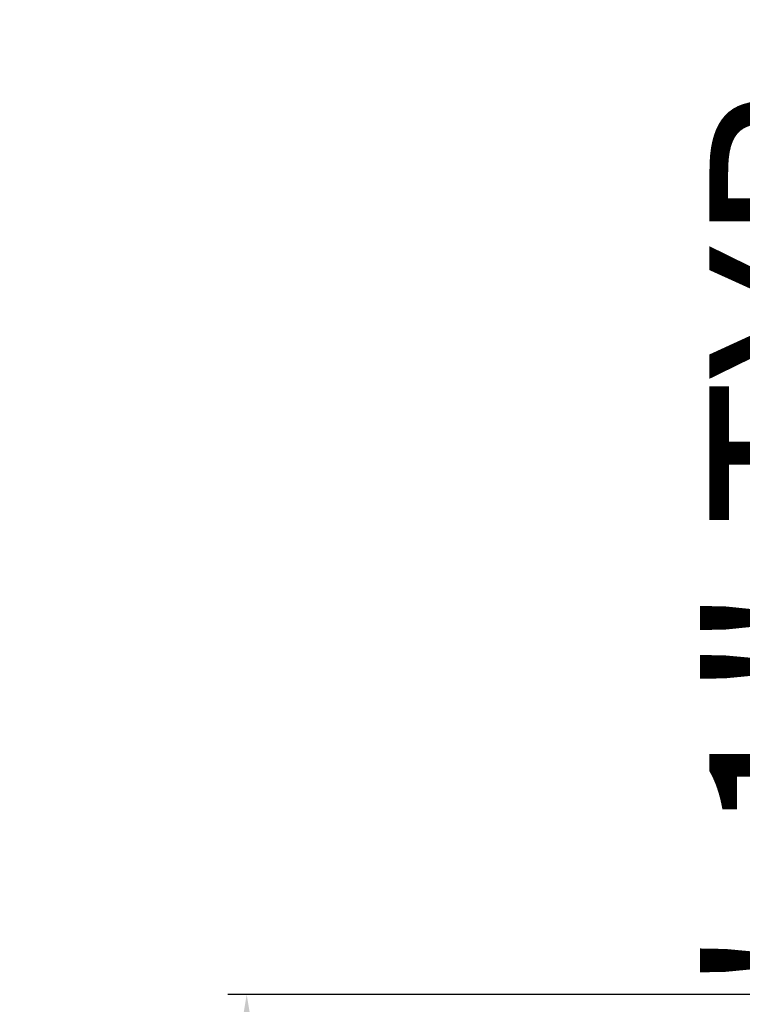
# Model space of a CAD drawing. Units: inches. Extents: x 2083 to 3317, y 1141 to 2115.
# Tile 21 of 256: x 2178 to 2226, y 1477 to 1542. Entities that reach past the tile are written whole.
import ezdxf

# ---------------------------------------------------------------- set-up
doc = ezdxf.new("R2010")
doc.units = ezdxf.units.IN
doc.layers.add('A-ANNO-DIMS', color=2, linetype='Continuous', lineweight=18)
doc.styles.get("Standard").update_dxf_attribs({"font": 'arial.ttf'})
doc.dimstyles.new('ISO-25', dxfattribs={"dimtxt": 12, "dimasz": 12, "dimexe": 1.25, "dimexo": 0.625, "dimtad": 1, "dimlunit": 3, "dimtxsty": 'Standard', "dimcen": 2.5, "dimadec": 0, "dimazin": 0, "dimtfac": 1, "dimtmove": 0, "dimatfit": 3, "dimfxl": 1, "dimarcsym": 0})

# ---------------------------------------------------------------- blocks, each defined once
blk = doc.blocks.new('*D13')
at = {"layer": 'A-ANNO-DIMS', "color": 0, "lineweight": -2, "transparency": 16777216}
for p, q in [((2226.335, 1477.761), (2191.976, 1477.761)), ((2193.226, 1465.761), (2193.226, 1275.261)), ((2226.335, 1263.261), (2191.976, 1263.261))]:
    blk.add_line(p, q, dxfattribs=at)
at = {"layer": 'A-ANNO-DIMS', "color": 0, "transparency": 16777216}
for points in [[(2191.226, 1465.761), (2195.226, 1465.761), (2193.226, 1477.761)], [(2191.226, 1275.261), (2195.226, 1275.261), (2193.226, 1263.261)]]:
    blk.add_solid(points, dxfattribs=at)
at = {"layer": 'Defpoints', "color": 0, "transparency": 16777216}
for p in [(2226.96, 1477.761), (2193.226, 1263.261), (2226.96, 1263.261)]:
    blk.add_point(p, dxfattribs=at)
at = {"layer": 'A-ANNO-DIMS', "color": 0, "transparency": 16777216, "insert": (2186.474, 1370.511), "char_height": 12, "attachment_point": 5, "rotation": 90}
blk.add_mtext('17\'-10.5"', dxfattribs=at)
blk = doc.blocks.new('*D30')
at = {"layer": 'A-ANNO-DIMS', "color": 0, "lineweight": -2, "transparency": 16777216}
for p, q in [((2240.018, 1445.274), (2240.018, 1448.046)), ((2254.329, 1445.274), (2254.329, 1448.046)), ((2228.018, 1446.796), (2216.018, 1446.796)), ((2240.018, 1446.796), (2254.329, 1446.796)), ((2266.329, 1446.796), (2413.765, 1446.796))]:
    blk.add_line(p, q, dxfattribs=at)
at = {"layer": 'A-ANNO-DIMS', "color": 0, "transparency": 16777216}
for points in [[(2228.018, 1448.796), (2228.018, 1444.796), (2240.018, 1446.796)], [(2266.329, 1448.796), (2266.329, 1444.796), (2254.329, 1446.796)]]:
    blk.add_solid(points, dxfattribs=at)
at = {"layer": 'Defpoints', "color": 0, "transparency": 16777216}
for p in [(2254.329, 1446.796), (2240.018, 1444.649), (2254.329, 1444.649)]:
    blk.add_point(p, dxfattribs=at)
at = {"layer": 'A-ANNO-DIMS', "color": 0, "transparency": 16777216, "insert": (2346.047, 1453.625), "char_height": 12, "attachment_point": 5}
blk.add_mtext('WC 1\'-2 1/2" TYP.', dxfattribs=at)
blk = doc.blocks.new('*D31')
at = {"layer": 'A-ANNO-DIMS', "color": 0, "lineweight": -2, "transparency": 16777216}
for p, q in [((2237.871, 1456.649), (2237.871, 1541.915)), ((2239.393, 1444.649), (2236.621, 1444.649)), ((2237.871, 1431.548), (2237.871, 1444.649)), ((2239.393, 1431.548), (2236.621, 1431.548)), ((2237.871, 1419.548), (2237.871, 1407.548))]:
    blk.add_line(p, q, dxfattribs=at)
at = {"layer": 'A-ANNO-DIMS', "color": 0, "transparency": 16777216}
for points in [[(2235.871, 1456.649), (2239.871, 1456.649), (2237.871, 1444.649)], [(2235.871, 1419.548), (2239.871, 1419.548), (2237.871, 1431.548)]]:
    blk.add_solid(points, dxfattribs=at)
at = {"layer": 'Defpoints', "color": 0, "transparency": 16777216}
for p in [(2237.871, 1444.649), (2240.018, 1444.649), (2240.018, 1431.548)]:
    blk.add_point(p, dxfattribs=at)
at = {"layer": 'A-ANNO-DIMS', "color": 0, "transparency": 16777216, "insert": (2231.217, 1505.282), "char_height": 12, "attachment_point": 5, "rotation": 90}
blk.add_mtext('1\'-1" TYP.', dxfattribs=at)

msp = doc.modelspace()

# ---------------------------------------------------------------- dimensions: what is measured, and where the dimension line sits
at = {"layer": 'A-ANNO-DIMS'}
dim = msp.add_linear_dim(base=(2237.871, 1444.649), p1=(2240.018, 1431.548), p2=(2240.018, 1444.649), angle=90, text='<> TYP.', dimstyle='ISO-25', override={"dimdec": 1, "dimlfac": 1, "dimrnd": 0, "dimzin": 1, "dimdsep": 46, "dimlunit": 4, "dimfrac": 2}, dxfattribs=at)
dim.commit()
dim.dimension.update_dxf_attribs({"geometry": '*D31', "text_midpoint": (2231.217, 1505.282)})
dim = msp.add_linear_dim(base=(2254.329, 1446.796), p1=(2240.018, 1444.649), p2=(2254.329, 1444.649), text='WC <> TYP.', dimstyle='ISO-25', override={"dimdec": 1, "dimlfac": 1, "dimrnd": 0, "dimzin": 1, "dimdsep": 46, "dimlunit": 4, "dimfrac": 2}, dxfattribs=at)
dim.commit()
dim.dimension.update_dxf_attribs({"geometry": '*D30', "text_midpoint": (2346.047, 1453.625)})
dim = msp.add_linear_dim(base=(2193.226, 1263.261), p1=(2226.96, 1477.761), p2=(2226.96, 1263.261), angle=90, dimstyle='ISO-25', override={"dimclrd": 0, "dimclre": 0, "dimclrt": 0}, dxfattribs=at)
dim.commit()
dim.dimension.update_dxf_attribs({"geometry": '*D13', "text_midpoint": (2186.474, 1370.511)})

doc.saveas('drawing.dxf')
